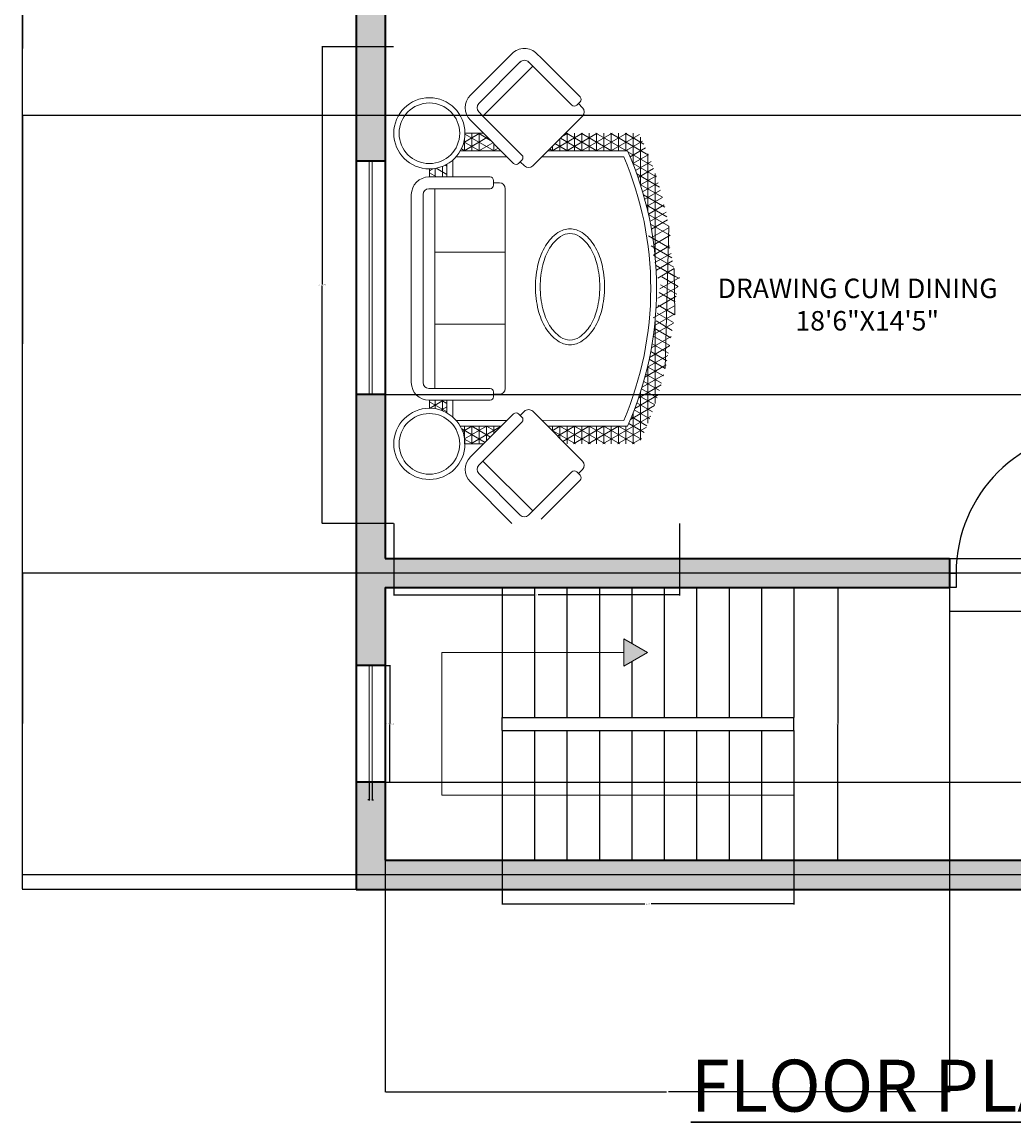
# Model space of a CAD drawing. Units: inches. Extents: x 5716 to 6907, y 12769 to 13594.
# Tile 1 of 17: x 5716 to 6022, y 12769 to 13109. Entities that reach past the tile are written whole.
import ezdxf

# ---------------------------------------------------------------- set-up
doc = ezdxf.new("R2010")
doc.units = ezdxf.units.IN
for name, color, linetype, lineweight in [('A-ANNO-DIMS', 2, 'Continuous', 18), ('A-ANNO-SYMB', 7, 'Continuous', 18), ('A-ANNO-TEXT', 7, 'Continuous', 30), ('A-AREA-IDEN', 7, 'Continuous', 18), ('A-DOOR', 4, 'Continuous', 25), ('A-FLOR-STRS', 7, 'Continuous', 25), ('A-FURN', 8, 'Continuous', 18), ('A-GLAZ', 4, 'Continuous', 18), ('A-WALL', 7, 'Continuous', 35), ('A-WALL-PATT', 252, 'Continuous', 13)]:
    doc.layers.add(name, color=color, linetype=linetype, lineweight=lineweight)
doc.styles.get("Standard").update_dxf_attribs({"font": 'arial.ttf'})
doc.dimstyles.get("Standard").update_dxf_attribs({"dimtxt": 0.18, "dimasz": 0.18, "dimexe": 0.18, "dimexo": 0.0625, "dimgap": 0.09, "dimtad": 0, "dimtih": 1, "dimtoh": 1, "dimdec": 4, "dimzin": 0, "dimdsep": 46, "dimtxsty": 'Standard', "dimcen": 0.09, "dimadec": 0, "dimazin": 0, "dimtfac": 1, "dimtdec": 4, "dimtofl": 0, "dimtmove": 0, "dimatfit": 3, "dimfxl": 1, "dimtolj": 1, "dimtzin": 0, "dimarcsym": 0})

# ---------------------------------------------------------------- blocks, each defined once
blk = doc.blocks.new('A$C7A76439A')
for p, q in [((2799, 2281.9), (1199, 2281.9)), ((1199, 2181.9), (2799, 2181.9)), ((948.9, 1978.3), (1035.6, 2128.3)), ((976.5, 2079.8), (1049, 2079.8)), ((1049, 2008), (979.5, 2128.3)), ((1049, 2128.3), (980.4, 2128.3)), ((1049, 2131.9), (1049, 2081.9)), ((1049, 2081.9), (1049, 1611.9)), ((1149, 1611.9), (1149, 2131.9)), ((2849, 2081.9), (1149, 2081.9)), ((1695.1, 2081.9), (1695.1, 1481.9)), ((2307.6, 2081.9), (2307.6, 1481.9)), ((2849, 2131.9), (2849, 1611.9)), ((2949, 2081.9), (2949, 2131.9)), ((3017.6, 2128.3), (2949, 2128.3)), ((2949, 2067.5), (2984.1, 2128.3)), ((2949, 1611.9), (2949, 2081.9)), ((2949, 2079.8), (3021.5, 2079.8)), ((2969.7, 1978.3), (3023.1, 2070.8)), ((3019.4, 2095.1), (3000.2, 2128.3)), ((940.7, 1978.3), (1049, 1978.3)), ((959.3, 2017.3), (1049, 2017.3)), ((993.9, 1978.3), (964, 2030.1)), ((1021.1, 1978.3), (1049, 2026.6)), ((2949, 2017.3), (3038.7, 2017.3)), ((2949, 1978.3), (3057.3, 1978.3)), ((3041.8, 1978.3), (3049.9, 1992.2)), ((877.3, 1467), (877.3, 1900.7)), ((905, 1928.3), (1049, 1928.3)), ((2949, 1928.3), (3093, 1928.3)), ((3120.6, 1900.7), (3120.6, 1467)), ((677.3, 1829.8), (827.3, 1829.8)), ((677.3, 1757.9), (717.8, 1828)), ((677.3, 1825.3), (677.3, 1667)), ((689.8, 1654.5), (804.6, 1853.3)), ((827.3, 1641.9), (719.7, 1828.3)), ((827.3, 1766.9), (782.7, 1844.2)), ((827.3, 1517), (827.3, 1865)), ((3170.6, 1865), (3170.6, 1517)), ((3170.6, 1826.4), (3187.7, 1856)), ((3170.6, 1701.4), (3247.3, 1834.3)), ((3286.4, 1632.8), (3170.6, 1833.2)), ((3170.6, 1829.8), (3268.5, 1829.8)), ((3170.6, 1576.4), (3314.4, 1825.4)), ((3320.6, 1698.4), (3241.3, 1835.9)), ((3320.6, 1823.4), (3319.5, 1825.3)), ((3320.6, 1667), (3320.6, 1825.3)), ((353.6, 1778.7), (0, 1425.1)), ((70.7, 1354.4), (424.3, 1708)), ((530.3, 1672.6), (495, 1708)), ((601, 1743.3), (565.7, 1778.7)), ((933.4, 1411), (601, 1743.3)), ((827.3, 1516.9), (677.3, 1776.7)), ((677.3, 1767.3), (827.3, 1767.3)), ((677.3, 1704.8), (827.3, 1704.8)), ((735.6, 1608.8), (827.3, 1767.7)), ((3064.6, 1411), (3396.9, 1743.3)), ((3170.6, 1767.3), (3320.6, 1767.3)), ((3240.6, 1587), (3170.6, 1708.2)), ((3170.6, 1704.8), (3320.6, 1704.8)), ((3260.3, 1606.7), (3320.6, 1711.2)), ((3396.9, 1743.3), (3432.3, 1778.7)), ((3467.6, 1672.6), (3503, 1708)), ((3927.3, 1354.4), (3573.7, 1708)), ((3644.4, 1778.7), (3998, 1425.1)), ((106.1, 1248.4), (530.3, 1672.6)), ((862.7, 1340.3), (530.3, 1672.6)), ((702.1, 1642.3), (827.3, 1642.3)), ((781.3, 1563), (827.3, 1642.7)), ((3135.3, 1340.3), (3467.6, 1672.6)), ((3891.9, 1248.4), (3467.6, 1672.6)), ((764.6, 1579.8), (827.3, 1579.8)), ((1099, 1581.9), (1079, 1581.9)), ((1119, 1581.9), (1099, 1581.9)), ((1099, 1581.9), (1099, 1531.9)), ((2899, 1581.9), (2879, 1581.9)), ((2919, 1581.9), (2899, 1581.9)), ((2899, 1581.9), (2899, 1531.9)), ((3194.9, 1541.3), (3170.6, 1583.2)), ((3170.6, 1579.8), (3233.4, 1579.8)), ((3170.6, 1517.3), (3170.9, 1517.3)), ((2849, 1481.9), (1149, 1481.9)), ((905.1, 1340.3), (933.4, 1368.6)), ((919.2, 1354.4), (954.6, 1319.1)), ((3078.7, 1354.4), (3043.4, 1319.1)), ((3092.9, 1340.3), (3064.6, 1368.6)), ((106.1, 1248.4), (70.7, 1283.7)), ((438.4, 916), (106.1, 1248.4)), ((530.3, 824.1), (954.6, 1248.4)), ((3467.6, 824.1), (3043.4, 1248.4)), ((3559.6, 916), (3891.9, 1248.4)), ((3891.9, 1248.4), (3927.3, 1283.7)), ((367.7, 845.3), (35.4, 1177.7)), ((877.3, 473.7), (879.6, 1173.4)), ((3120.6, 1171.1), (3120.6, 473.7)), ((3630.3, 845.3), (3962.6, 1177.7)), ((3998, 1213), (3962.6, 1177.7)), ((677.3, 882.9), (797.8, 1091.6)), ((827.3, 891.9), (743.4, 1037.2)), ((786, 1079.8), (827.3, 1079.8)), ((827.3, 1016.9), (789.2, 1083)), ((827.3, 440.9), (827.3, 1121.1)), ((3170.6, 1121.1), (3170.6, 440.9)), ((3170.6, 1076.4), (3187, 1104.8)), ((3320.6, 823.4), (3170.6, 1083.2)), ((3170.6, 1079.8), (3211.9, 1079.8)), ((3170.6, 951.4), (3232.8, 1059)), ((677.3, 757.9), (827.3, 1017.7)), ((677.3, 954.8), (827.3, 954.8)), ((827.3, 766.9), (697.7, 991.5)), ((723.5, 1017.3), (827.3, 1017.3)), ((3170.6, 1017.3), (3274.4, 1017.3)), ((3170.6, 826.4), (3278.5, 1013.2)), ((3170.6, 701.4), (3320.6, 961.2)), ((3320.6, 698.4), (3170.6, 958.2)), ((3170.6, 954.8), (3320.6, 954.8)), ((3320.6, 948.4), (3289.6, 1002.1)), ((410.1, 845.3), (438.4, 873.6)), ((424.3, 859.5), (459.6, 824.1)), ((827.3, 641.9), (677.3, 901.7)), ((677.3, 632.9), (827.3, 892.7)), ((677.3, 892.3), (827.3, 892.3)), ((3170.6, 892.3), (3320.6, 892.3)), ((3573.7, 859.5), (3538.4, 824.1)), ((3587.9, 845.3), (3559.6, 873.6)), ((677.3, 829.8), (827.3, 829.8)), ((827.3, 516.9), (677.3, 776.7)), ((677.3, 507.9), (827.3, 767.7)), ((677.3, 767.3), (827.3, 767.3)), ((3170.6, 576.4), (3320.6, 836.2)), ((3320.6, 573.4), (3170.6, 833.2)), ((3170.6, 829.8), (3320.6, 829.8)), ((3170.6, 767.3), (3320.6, 767.3)), ((677.3, 704.8), (827.3, 704.8)), ((3170.6, 451.4), (3320.6, 711.2)), ((3320.6, 448.4), (3170.6, 708.2)), ((3170.6, 704.8), (3320.6, 704.8)), ((913, 243.6), (677.3, 651.7)), ((677.3, 382.9), (827.3, 642.7)), ((677.3, 642.3), (827.3, 642.3)), ((677.3, 579.8), (827.3, 579.8)), ((3133.8, 262.7), (3320.6, 586.2)), ((3170.6, 642.3), (3320.6, 642.3)), ((3310.9, 340.3), (3170.6, 583.2)), ((3170.6, 579.8), (3320.6, 579.8)), ((819.1, 281.2), (677.3, 526.7)), ((677.3, 517.3), (827.3, 517.3)), ((716.8, 326.3), (827.3, 517.7)), ((3170.6, 517.3), (3320.6, 517.3)), ((677.3, 454.8), (827.3, 454.8)), ((722.3, 323.8), (677.3, 401.7)), ((677.3, 392.3), (944.2, 392.3)), ((774.1, 300.5), (849.6, 431.2)), ((832, 275.8), (907.7, 406.9)), ((1004.3, 210.4), (885.6, 415.9)), ((890.6, 252.2), (966.5, 383.7)), ((1093.3, 181.2), (979.2, 378.9)), ((2951, 196.1), (3067.5, 397.7)), ((3041.2, 227.3), (3162.5, 437.4)), ((3053.8, 392.3), (3320.6, 392.3)), ((3138.2, 264.4), (3062.4, 395.7)), ((3196.4, 288.6), (3120.8, 419.5)), ((3254, 313.9), (3170.6, 458.2)), ((3170.6, 454.8), (3320.6, 454.8)), ((3229.2, 302.8), (3320.6, 461.2)), ((709.3, 329.8), (1120.8, 329.8)), ((949.8, 229.8), (1026, 361.8)), ((1009.7, 208.6), (1086.2, 341.1)), ((1180.3, 155.6), (1070.1, 346.5)), ((1070.3, 188.5), (1147.1, 321.6)), ((1131.5, 169.6), (1208.8, 303.4)), ((1265.4, 133.2), (1158.6, 318.1)), ((1193.5, 151.9), (1271.2, 286.4)), ((1348.8, 113.7), (1245.1, 293.3)), ((2610.1, 105.5), (2712.4, 282.8)), ((2692.7, 123.6), (2797.9, 305.9)), ((2837, 161), (2759.6, 295.2)), ((2776.9, 144.5), (2885.5, 332.5)), ((2898.6, 179.3), (2821.6, 312.8)), ((2863, 168.6), (2975.2, 362.9)), ((2877.1, 329.8), (3288.7, 329.8)), ((2959.5, 198.9), (2882.9, 331.6)), ((3019.7, 219.6), (2943.4, 351.8)), ((3079.3, 241.4), (3003.3, 373.1)), ((852.7, 267.3), (1349.4, 267.3)), ((1020.7, 204.8), (1744.2, 204.8)), ((1256.2, 135.5), (1334.3, 270.8)), ((1319.6, 120.3), (1398.2, 256.5)), ((1430.6, 97), (1329.6, 271.9)), ((1383.7, 106.3), (1462.9, 243.6)), ((1510.9, 82.9), (1412.4, 253.6)), ((1448.6, 93.7), (1528.4, 232)), ((1589.9, 71.2), (1493.6, 238)), ((1514.2, 82.4), (1594.8, 221.9)), ((1580.6, 72.4), (1661.9, 213.2)), ((1705.7, 49.7), (1607.2, 220.4)), ((1643.3, 60.5), (1723.2, 198.8)), ((1784.6, 38), (1688.3, 204.8)), ((1709, 49.2), (1789.5, 188.7)), ((1852.3, 42.6), (1748.6, 222.2)), ((1934.2, 25.9), (1833.2, 200.8)), ((2100.1, 34.3), (2197.6, 203.1)), ((2234.3, 57.4), (2154.8, 195.2)), ((2179.8, 47.3), (2279.6, 220.1)), ((2298.8, 70.8), (2219.9, 207.5)), ((2253.8, 204.8), (2977.3, 204.8)), ((2260.9, 62.8), (2363.3, 240.1)), ((2362.6, 85.4), (2284.2, 221.1)), ((2343.5, 80.9), (2448.8, 263.2)), ((2452.3, 77.5), (2371.4, 217.6)), ((2518.3, 88.1), (2438.1, 227)), ((2449.3, 77), (2546.8, 245.8)), ((2583.5, 100.1), (2504, 237.9)), ((2529, 90), (2628.7, 262.8)), ((2648, 113.5), (2569, 250.2)), ((2711.7, 128.1), (2633.3, 263.8)), ((2648.6, 267.3), (3145.3, 267.3)), ((2774.7, 143.9), (2696.8, 278.8)), ((1319.6, 120.3), (2529, 90)), ((1775.4, 39.2), (1856.7, 180)), ((1887.2, 35.2), (1966.5, 172.4)), ((2014.5, 11.7), (1916, 182.4)), ((1952.1, 22.5), (2032, 160.9)), ((2093.4, 0), (1997.1, 166.8)), ((2017.8, 11.2), (2098.3, 150.7)), ((2084.2, 1.3), (2165.5, 142.1)), ((2169.1, 45.4), (2088.9, 184.3)), ((1775.4, 39.2), (2169.1, 45.4))]:
    blk.add_line(p, q)
for centre, radius in [((677.3, 2128.3), 303), ((677.3, 2128.3), 258), ((3320.6, 2128.3), 303), ((3320.6, 2128.3), 258)]:
    blk.add_circle(centre, radius)
for centre, radius, start, end in [((1199, 2131.9), 150, 90, 180), ((2799, 2131.9), 150, 0, 90), ((1199, 2131.9), 50, 90, 180), ((2799, 2131.9), 50, 0, 90), ((459.6, 1672.6), 150, 45, 135), ((3538.4, 1672.6), 150, 45, 135), ((459.6, 1672.6), 50, 45, 135), ((3538.4, 1672.6), 50, 45, 135), ((1079, 1611.9), 30, 180, 270), ((1119, 1611.9), 30, 270, 0), ((2879, 1611.9), 30, 180, 270), ((2919, 1611.9), 30, 270, 0), ((1149, 1531.9), 50, 180, 270), ((2849, 1531.9), 50, 270, 0), ((912.2, 1389.8), 30, 315, 45), ((3085.8, 1389.8), 30, 135, 225), ((3891.9, 1319.1), 150, 315, 45), ((106.1, 1319.1), 50, 135, 225), ((883.9, 1361.5), 30, 225, 315), ((919.2, 1283.7), 50, 315, 45), ((3078.7, 1283.7), 50, 135, 225), ((3114.1, 1361.5), 30, 225, 315), ((3891.9, 1319.1), 50, 315, 45), ((2014.2, 399.9), 825, 90, 103.86382), ((2014.2, 399.9), 825, 76.13618, 90), ((1850.9, 827.5), 362.5, 120.78817, 145.1939), ((1949.5, 662.2), 555, 103.86382, 120.78817), ((1949.5, 662.2), 515, 103.86382, 120.78817), ((2014.2, 399.9), 785, 90, 103.86382), ((2014.2, 399.9), 785, 76.13618, 90), ((2078.9, 662.2), 515, 59.21183, 76.13618), ((2078.9, 662.2), 555, 59.21183, 76.13618), ((2177.4, 827.5), 362.5, 34.8061, 59.21183), ((1702, 931.1), 181, 145.1939, 180), ((1850.9, 827.5), 322.5, 120.78817, 145.1939), ((2177.4, 827.5), 322.5, 34.8061, 59.21183), ((2326.4, 931.1), 181, 0, 34.8061), ((1702, 931.1), 141, 145.1939, 180), ((2326.4, 931.1), 141, 0, 34.8061), ((388.9, 866.5), 30, 225, 315), ((417.2, 894.8), 30, 315, 45), ((1702, 931.1), 181, 180, 214.8061), ((1702, 931.1), 141, 180, 214.8061), ((1850.9, 1034.6), 322.5, 214.8061, 239.21183), ((2177.4, 1034.6), 322.5, 300.78817, 325.1939), ((2326.4, 931.1), 141, 325.1939, 0), ((2326.4, 931.1), 181, 325.1939, 0), ((3580.8, 894.8), 30, 135, 225), ((3609.1, 866.5), 30, 225, 315), ((495, 859.5), 50, 225, 315), ((1850.9, 1034.6), 362.5, 214.8061, 239.21183), ((1949.5, 1200), 515, 239.21183, 256.13618), ((2078.9, 1200), 515, 283.86382, 300.78817), ((2177.4, 1034.6), 362.5, 300.78817, 325.1939), ((3503, 859.5), 50, 225, 315), ((1949.5, 1200), 555, 239.21183, 256.13618), ((2014.2, 1462.2), 825, 256.13618, 270), ((2014.2, 1462.2), 785, 256.13618, 270), ((2014.2, 1462.2), 785, 270, 283.86382), ((2014.2, 1462.2), 825, 270, 283.86382), ((2078.9, 1200), 555, 283.86382, 300.78817), ((1999, 3092.2), 2848.7, 246.81236, 293.18764), ((1999, 3092.2), 2898.7, 246.15892, 293.84108)]:
    blk.add_arc(centre, radius, start, end)
blk = doc.blocks.new('DOOR-SWING-48IN')
for p, q in [((-2, 43.95), (-2, 0)), ((0, 44), (0, 0)), ((-46, 0), (-44, 0)), ((-44, 0), (-44, -4.5)), ((0, 0), (-2, 0)), ((2, 0), (0, 0)), ((0, 0), (0, -4.5)), ((-44, -4.5), (-46, -4.5)), ((0, -4.5), (2, -4.5))]:
    blk.add_line(p, q)
blk.add_arc((0, 0), 44, 90, 180)
blk = doc.blocks.new('WIN-GLAZING-72IN')
for p, q in [((0, 0), (0, -72)), ((1, 0), (1, -72))]:
    blk.add_line(p, q)
blk = doc.blocks.new('WIN-GLAZING-36IN')
for p, q in [((0, 0), (0, 36)), ((1, 0), (1, 36))]:
    blk.add_line(p, q)
blk = doc.blocks.new('STAIR-RETURN-FLIGHT')
for p, q in [((0, 84), (0, 44)), ((10, 84), (10, 44)), ((20, 84), (20, 44)), ((30, 84), (30, 44)), ((40, 84), (40, 66.79)), ((50, 84), (50, 44)), ((60, 84), (60, 44)), ((70, 84), (70, 44)), ((80, 84), (80, 44)), ((90, 84), (90, 44)), ((40, 61.21), (40, 44)), ((0, 44), (90, 44)), ((0, 40), (0, 44)), ((90, 40), (90, 44)), ((0, 40), (90, 40)), ((0, 40), (0, 0)), ((10, 40), (10, 0)), ((20, 40), (20, 0)), ((30, 40), (30, 0)), ((40, 40), (40, 0)), ((50, 40), (50, 0)), ((60, 40), (60, 0)), ((70, 40), (70, 0)), ((80, 40), (80, 0)), ((90, 40), (90, 0))]:
    blk.add_line(p, q)
blk = doc.blocks.new('*D33')
at = {"layer": 'A-ANNO-DIMS', "color": 0, "lineweight": -2, "transparency": 16777216}
for p, q in [((5830.57, 13100.85), (5808.41, 13100.85)), ((5808.59, 13100.67), (5808.59, 13027.58)), ((5808.59, 12954.12), (5808.59, 13027.21)), ((5830.57, 12953.94), (5808.41, 12953.94))]:
    blk.add_line(p, q, dxfattribs=at)
at = {"layer": 'A-ANNO-DIMS', "color": 0, "transparency": 16777216}
for points in [[(5808.56, 13100.67), (5808.62, 13100.67), (5808.59, 13100.85)], [(5808.56, 12954.12), (5808.62, 12954.12), (5808.59, 12953.94)]]:
    blk.add_solid(points, dxfattribs=at)
at = {"layer": 'Defpoints', "color": 0, "transparency": 16777216}
for p in [(5808.59, 13100.85), (5830.63, 13100.85), (5830.63, 12953.94)]:
    blk.add_point(p, dxfattribs=at)
at = {"layer": 'A-ANNO-DIMS', "color": 0, "transparency": 16777216, "insert": (5808.59, 13027.4), "char_height": 0.18, "attachment_point": 5}
blk.add_mtext('\\A1;SOFA GROUP 147 TYP.', dxfattribs=at)
blk = doc.blocks.new('*D34')
at = {"layer": 'A-ANNO-DIMS', "color": 0, "lineweight": -2, "transparency": 16777216}
for p, q in [((5830.63, 12953.88), (5830.63, 12931.72)), ((5918.69, 12953.88), (5918.69, 12931.72)), ((5830.81, 12931.9), (5874.13, 12931.9)), ((5918.51, 12931.9), (5875.19, 12931.9))]:
    blk.add_line(p, q, dxfattribs=at)
at = {"layer": 'A-ANNO-DIMS', "color": 0, "transparency": 16777216}
for points in [[(5830.81, 12931.93), (5830.81, 12931.87), (5830.63, 12931.9)], [(5918.51, 12931.93), (5918.51, 12931.87), (5918.69, 12931.9)]]:
    blk.add_solid(points, dxfattribs=at)
at = {"layer": 'Defpoints', "color": 0, "transparency": 16777216}
for p in [(5830.63, 12953.94), (5918.69, 12953.94), (5830.63, 12931.9)]:
    blk.add_point(p, dxfattribs=at)
at = {"layer": 'A-ANNO-DIMS', "color": 0, "transparency": 16777216, "insert": (5874.66, 12931.9), "char_height": 0.18, "attachment_point": 5}
blk.add_mtext('\\A1;88 TYP.', dxfattribs=at)
blk = doc.blocks.new('*D42')
at = {"layer": 'A-ANNO-DIMS', "color": 0, "lineweight": -2, "transparency": 16777216}
for p, q in [((6002.02, 12934.09), (6002.02, 12926.69)), ((6050.02, 12934.09), (6050.02, 12926.69)), ((6002.2, 12926.87), (6025.49, 12926.87)), ((6049.84, 12926.87), (6026.55, 12926.87))]:
    blk.add_line(p, q, dxfattribs=at)
at = {"layer": 'A-ANNO-DIMS', "color": 0, "transparency": 16777216}
for points in [[(6002.2, 12926.9), (6002.2, 12926.84), (6002.02, 12926.87)], [(6049.84, 12926.9), (6049.84, 12926.84), (6050.02, 12926.87)]]:
    blk.add_solid(points, dxfattribs=at)
at = {"layer": 'Defpoints', "color": 0, "transparency": 16777216}
for p in [(6002.02, 12934.15), (6050.02, 12934.15), (6050.02, 12926.87)]:
    blk.add_point(p, dxfattribs=at)
at = {"layer": 'A-ANNO-DIMS', "color": 0, "transparency": 16777216, "insert": (6026.02, 12926.87), "char_height": 0.18, "attachment_point": 5}
blk.add_mtext('\\A1;48 TYP.', dxfattribs=at)
blk = doc.blocks.new('*D43')
at = {"layer": 'A-ANNO-DIMS', "color": 0, "lineweight": -2, "transparency": 16777216}
for p, q in [((5824.09, 12910.15), (5829.6, 12910.15)), ((5829.42, 12909.97), (5829.42, 12892.33)), ((5829.42, 12874.33), (5829.42, 12891.97)), ((5824.09, 12874.15), (5829.6, 12874.15))]:
    blk.add_line(p, q, dxfattribs=at)
at = {"layer": 'A-ANNO-DIMS', "color": 0, "transparency": 16777216}
for points in [[(5829.39, 12909.97), (5829.45, 12909.97), (5829.42, 12910.15)], [(5829.39, 12874.33), (5829.45, 12874.33), (5829.42, 12874.15)]]:
    blk.add_solid(points, dxfattribs=at)
at = {"layer": 'Defpoints', "color": 0, "transparency": 16777216}
for p in [(5824.02, 12910.15), (5829.42, 12910.15), (5824.02, 12874.15)]:
    blk.add_point(p, dxfattribs=at)
at = {"layer": 'A-ANNO-DIMS', "color": 0, "transparency": 16777216, "insert": (5829.42, 12892.15), "char_height": 0.18, "attachment_point": 5}
blk.add_mtext('\\A1;STAIR WINDOW 36 TYP.', dxfattribs=at)
blk = doc.blocks.new('*D44')
at = {"layer": 'A-ANNO-DIMS', "color": 0, "lineweight": -2, "transparency": 16777216}
for p, q in [((5823.02, 12874.09), (5823.02, 12868.57)), ((5824.02, 12874.09), (5824.02, 12868.57)), ((5822.84, 12868.75), (5822.66, 12868.75)), ((5824.2, 12868.75), (5824.38, 12868.75))]:
    blk.add_line(p, q, dxfattribs=at)
at = {"layer": 'A-ANNO-DIMS', "color": 0, "transparency": 16777216}
for points in [[(5822.84, 12868.78), (5822.84, 12868.72), (5823.02, 12868.75)], [(5824.2, 12868.78), (5824.2, 12868.72), (5824.02, 12868.75)]]:
    blk.add_solid(points, dxfattribs=at)
at = {"layer": 'Defpoints', "color": 0, "transparency": 16777216}
for p in [(5823.02, 12874.15), (5824.02, 12874.15), (5824.02, 12868.75)]:
    blk.add_point(p, dxfattribs=at)
at = {"layer": 'A-ANNO-DIMS', "color": 0, "transparency": 16777216, "insert": (5823.52, 12868.75), "char_height": 0.18, "attachment_point": 5}
blk.add_mtext('\\A1;1 TYP.', dxfattribs=at)
blk = doc.blocks.new('*D45')
at = {"layer": 'A-ANNO-DIMS', "color": 0, "lineweight": -2, "transparency": 16777216}
for p, q in [((5864.02, 12850.09), (5864.02, 12836.47)), ((5954.02, 12850.09), (5954.02, 12836.47)), ((5864.2, 12836.65), (5908.09, 12836.65)), ((5953.84, 12836.65), (5909.96, 12836.65))]:
    blk.add_line(p, q, dxfattribs=at)
at = {"layer": 'A-ANNO-DIMS', "color": 0, "transparency": 16777216}
for points in [[(5864.2, 12836.68), (5864.2, 12836.62), (5864.02, 12836.65)], [(5953.84, 12836.68), (5953.84, 12836.62), (5954.02, 12836.65)]]:
    blk.add_solid(points, dxfattribs=at)
at = {"layer": 'Defpoints', "color": 0, "transparency": 16777216}
for p in [(5864.02, 12850.15), (5954.02, 12850.15), (5954.02, 12836.65)]:
    blk.add_point(p, dxfattribs=at)
at = {"layer": 'A-ANNO-DIMS', "color": 0, "transparency": 16777216, "insert": (5909.02, 12836.65), "char_height": 0.18, "attachment_point": 5}
blk.add_mtext('\\A1;STAIR 90 TYP.', dxfattribs=at)
blk = doc.blocks.new('*D46')
at = {"layer": 'A-ANNO-DIMS', "color": 0, "lineweight": -2, "transparency": 16777216}
for p, q in [((5954.09, 12934.15), (5967.7, 12934.15)), ((5967.52, 12933.97), (5967.52, 12892.33)), ((5967.52, 12850.33), (5967.52, 12891.97)), ((5954.09, 12850.15), (5967.7, 12850.15))]:
    blk.add_line(p, q, dxfattribs=at)
at = {"layer": 'A-ANNO-DIMS', "color": 0, "transparency": 16777216}
for points in [[(5967.49, 12933.97), (5967.55, 12933.97), (5967.52, 12934.15)], [(5967.49, 12850.33), (5967.55, 12850.33), (5967.52, 12850.15)]]:
    blk.add_solid(points, dxfattribs=at)
at = {"layer": 'Defpoints', "color": 0, "transparency": 16777216}
for p in [(5954.02, 12934.15), (5967.52, 12934.15), (5954.02, 12850.15)]:
    blk.add_point(p, dxfattribs=at)
at = {"layer": 'A-ANNO-DIMS', "color": 0, "transparency": 16777216, "insert": (5967.52, 12892.15), "char_height": 0.18, "attachment_point": 5}
blk.add_mtext('\\A1;84 TYP.', dxfattribs=at)
blk = doc.blocks.new('*D50')
at = {"layer": 'A-ANNO-DIMS', "color": 0, "lineweight": -2, "transparency": 16777216}
for p, q in [((5818.96, 13440.15), (5716.04, 13440.15)), ((5716.22, 13439.97), (5716.22, 13140.83)), ((5716.22, 12841.33), (5716.22, 13140.47)), ((5818.96, 12841.15), (5716.04, 12841.15))]:
    blk.add_line(p, q, dxfattribs=at)
at = {"layer": 'A-ANNO-DIMS', "color": 0, "transparency": 16777216}
for points in [[(5716.19, 13439.97), (5716.25, 13439.97), (5716.22, 13440.15)], [(5716.19, 12841.33), (5716.25, 12841.33), (5716.22, 12841.15)]]:
    blk.add_solid(points, dxfattribs=at)
at = {"layer": 'Defpoints', "color": 0, "transparency": 16777216}
for p in [(5716.22, 13440.15), (5819.02, 13440.15), (5819.02, 12841.15)]:
    blk.add_point(p, dxfattribs=at)
at = {"layer": 'A-ANNO-DIMS', "color": 0, "transparency": 16777216, "insert": (5716.22, 13140.65), "char_height": 0.18, "attachment_point": 5}
blk.add_mtext('\\A1;599', dxfattribs=at)
blk = doc.blocks.new('*D52')
at = {"layer": 'A-ANNO-DIMS', "color": 0, "lineweight": -2, "transparency": 16777216}
for p, q in [((6267.34, 13440.15), (5716.04, 13440.15)), ((5716.22, 13439.97), (5716.22, 13140.83)), ((5716.22, 12841.33), (5716.22, 13140.47)), ((6267.34, 12841.15), (5716.04, 12841.15))]:
    blk.add_line(p, q, dxfattribs=at)
at = {"layer": 'A-ANNO-DIMS', "color": 0, "transparency": 16777216}
for points in [[(5716.19, 13439.97), (5716.25, 13439.97), (5716.22, 13440.15)], [(5716.19, 12841.33), (5716.25, 12841.33), (5716.22, 12841.15)]]:
    blk.add_solid(points, dxfattribs=at)
at = {"layer": 'Defpoints', "color": 0, "transparency": 16777216}
for p in [(6267.41, 13440.15), (5716.22, 12841.15), (6267.41, 12841.15)]:
    blk.add_point(p, dxfattribs=at)
at = {"layer": 'A-ANNO-DIMS', "color": 0, "transparency": 16777216, "insert": (5716.22, 13140.65), "char_height": 0.18, "attachment_point": 5}
blk.add_mtext('\\A1;599', dxfattribs=at)
blk = doc.blocks.new('*D62')
at = {"layer": 'A-ANNO-DIMS', "color": 0, "lineweight": -2, "transparency": 16777216}
for p, q in [((6736.67, 13120.65), (5716.04, 13120.65)), ((5716.22, 13120.47), (5716.22, 13100.33)), ((5716.22, 13079.83), (5716.22, 13099.97)), ((6736.67, 13079.65), (5716.04, 13079.65))]:
    blk.add_line(p, q, dxfattribs=at)
at = {"layer": 'A-ANNO-DIMS', "color": 0, "transparency": 16777216}
for points in [[(5716.19, 13120.47), (5716.25, 13120.47), (5716.22, 13120.65)], [(5716.19, 13079.83), (5716.25, 13079.83), (5716.22, 13079.65)]]:
    blk.add_solid(points, dxfattribs=at)
at = {"layer": 'Defpoints', "color": 0, "transparency": 16777216}
for p in [(6736.73, 13120.65), (5716.22, 13079.65), (6736.73, 13079.65)]:
    blk.add_point(p, dxfattribs=at)
at = {"layer": 'A-ANNO-DIMS', "color": 0, "transparency": 16777216, "insert": (5716.22, 13100.15), "char_height": 0.18, "attachment_point": 5}
blk.add_mtext('\\A1;41', dxfattribs=at)
blk = doc.blocks.new('*D63')
at = {"layer": 'A-ANNO-DIMS', "color": 0, "lineweight": -2, "transparency": 16777216}
for p, q in [((6736.67, 13079.65), (5716.04, 13079.65)), ((5716.22, 13079.47), (5716.22, 13009.33)), ((5716.22, 12938.83), (5716.22, 13008.97)), ((6736.67, 12938.65), (5716.04, 12938.65))]:
    blk.add_line(p, q, dxfattribs=at)
at = {"layer": 'A-ANNO-DIMS', "color": 0, "transparency": 16777216}
for points in [[(5716.19, 13079.47), (5716.25, 13079.47), (5716.22, 13079.65)], [(5716.19, 12938.83), (5716.25, 12938.83), (5716.22, 12938.65)]]:
    blk.add_solid(points, dxfattribs=at)
at = {"layer": 'Defpoints', "color": 0, "transparency": 16777216}
for p in [(6736.73, 13079.65), (5716.22, 12938.65), (6736.73, 12938.65)]:
    blk.add_point(p, dxfattribs=at)
at = {"layer": 'A-ANNO-DIMS', "color": 0, "transparency": 16777216, "insert": (5716.22, 13009.15), "char_height": 0.18, "attachment_point": 5}
blk.add_mtext('\\A1;141', dxfattribs=at)
blk = doc.blocks.new('*D64')
at = {"layer": 'A-ANNO-DIMS', "color": 0, "lineweight": -2, "transparency": 16777216}
for p, q in [((6736.67, 12938.65), (5716.04, 12938.65)), ((5716.22, 12938.47), (5716.22, 12892.33)), ((5716.22, 12845.83), (5716.22, 12891.97)), ((6736.67, 12845.65), (5716.04, 12845.65))]:
    blk.add_line(p, q, dxfattribs=at)
at = {"layer": 'A-ANNO-DIMS', "color": 0, "transparency": 16777216}
for points in [[(5716.19, 12938.47), (5716.25, 12938.47), (5716.22, 12938.65)], [(5716.19, 12845.83), (5716.25, 12845.83), (5716.22, 12845.65)]]:
    blk.add_solid(points, dxfattribs=at)
at = {"layer": 'Defpoints', "color": 0, "transparency": 16777216}
for p in [(6736.73, 12938.65), (5716.22, 12845.65), (6736.73, 12845.65)]:
    blk.add_point(p, dxfattribs=at)
at = {"layer": 'A-ANNO-DIMS', "color": 0, "transparency": 16777216, "insert": (5716.22, 12892.15), "char_height": 0.18, "attachment_point": 5}
blk.add_mtext('\\A1;93', dxfattribs=at)
blk = doc.blocks.new('*D66')
at = {"layer": 'A-ANNO-DIMS', "color": 0, "lineweight": -2, "transparency": 16777216}
for p, q in [((6002.02, 12934.09), (6002.02, 12778.62)), ((5828.02, 12850.09), (5828.02, 12778.62)), ((5828.2, 12778.8), (5914.74, 12778.8)), ((6001.84, 12778.8), (5915.3, 12778.8))]:
    blk.add_line(p, q, dxfattribs=at)
at = {"layer": 'A-ANNO-DIMS', "color": 0, "transparency": 16777216}
for points in [[(5828.2, 12778.83), (5828.2, 12778.77), (5828.02, 12778.8)], [(6001.84, 12778.83), (6001.84, 12778.77), (6002.02, 12778.8)]]:
    blk.add_solid(points, dxfattribs=at)
at = {"layer": 'Defpoints', "color": 0, "transparency": 16777216}
for p in [(6002.02, 12934.15), (5828.02, 12850.15), (6002.02, 12778.8)]:
    blk.add_point(p, dxfattribs=at)
at = {"layer": 'A-ANNO-DIMS', "color": 0, "transparency": 16777216, "insert": (5915.02, 12778.8), "char_height": 0.18, "attachment_point": 5}
blk.add_mtext('\\A1;174', dxfattribs=at)
blk = doc.blocks.new('*D67')
at = {"layer": 'A-ANNO-DIMS', "color": 0, "lineweight": -2, "transparency": 16777216}
for p, q in [((5819.09, 12874.15), (6907.26, 12874.15)), ((6907.08, 12873.97), (6907.08, 12857.83)), ((6907.08, 12841.33), (6907.08, 12857.47)), ((5819.09, 12841.15), (6907.26, 12841.15))]:
    blk.add_line(p, q, dxfattribs=at)
at = {"layer": 'A-ANNO-DIMS', "color": 0, "transparency": 16777216}
for points in [[(6907.05, 12873.97), (6907.11, 12873.97), (6907.08, 12874.15)], [(6907.05, 12841.33), (6907.11, 12841.33), (6907.08, 12841.15)]]:
    blk.add_solid(points, dxfattribs=at)
at = {"layer": 'Defpoints', "color": 0, "transparency": 16777216}
for p in [(5819.02, 12874.15), (6907.08, 12874.15), (5819.02, 12841.15)]:
    blk.add_point(p, dxfattribs=at)
at = {"layer": 'A-ANNO-DIMS', "color": 0, "transparency": 16777216, "insert": (6907.08, 12857.65), "char_height": 0.18, "attachment_point": 5}
blk.add_mtext('\\A1;33', dxfattribs=at)
blk = doc.blocks.new('*D68')
at = {"layer": 'A-ANNO-DIMS', "color": 0, "lineweight": -2, "transparency": 16777216}
for p, q in [((5828.09, 12993.65), (6907.26, 12993.65)), ((6907.08, 12993.47), (6907.08, 12968.58)), ((6907.08, 12943.33), (6907.08, 12968.22)), ((5828.09, 12943.15), (6907.26, 12943.15))]:
    blk.add_line(p, q, dxfattribs=at)
at = {"layer": 'A-ANNO-DIMS', "color": 0, "transparency": 16777216}
for points in [[(6907.05, 12993.47), (6907.11, 12993.47), (6907.08, 12993.65)], [(6907.05, 12943.33), (6907.11, 12943.33), (6907.08, 12943.15)]]:
    blk.add_solid(points, dxfattribs=at)
at = {"layer": 'Defpoints', "color": 0, "transparency": 16777216}
for p in [(5828.02, 12993.65), (6907.08, 12993.65), (5828.02, 12943.15)]:
    blk.add_point(p, dxfattribs=at)
at = {"layer": 'A-ANNO-DIMS', "color": 0, "transparency": 16777216, "insert": (6907.08, 12968.4), "char_height": 0.18, "attachment_point": 5}
blk.add_mtext('\\A1;50.5', dxfattribs=at)

msp = doc.modelspace()

# ---------------------------------------------------------------- hatches: boundary and pattern name
at = {"layer": 'A-ANNO-SYMB'}
h = msp.add_hatch(color=256, dxfattribs=at)
h.dxf.hatch_style = 1
h.paths.add_polyline_path([(5901.6, 12909.96), (5908.86, 12914.15), (5901.6, 12918.34)])
at = {"layer": 'A-WALL-PATT'}
h = msp.add_hatch(color=256, dxfattribs=at)
h.dxf.hatch_style = 1
h.paths.add_polyline_path([(5900.02, 13125.15), (5828.02, 13125.15), (5828.02, 13149.15), (5819.02, 13149.15), (5819.02, 13065.65), (5828.02, 13065.65), (5828.02, 13116.15), (5900.02, 13116.15)])
h = msp.add_hatch(color=256, dxfattribs=at)
h.dxf.hatch_style = 1
h.paths.add_polyline_path([(6002.02, 12943.15), (5828.02, 12943.15), (5828.02, 12993.65), (5819.02, 12993.65), (5819.02, 12910.15), (5828.02, 12910.15), (5828.02, 12934.15), (6002.02, 12934.15)])
h = msp.add_hatch(color=256, dxfattribs=at)
h.dxf.hatch_style = 1
h.paths.add_polyline_path([(6059.02, 12862.15), (6050.02, 12862.15), (6050.02, 12850.15), (5828.02, 12850.15), (5828.02, 12874.15), (5819.02, 12874.15), (5819.02, 12841.15), (6059.02, 12841.15)])

# ---------------------------------------------------------------- linework, layer by layer
at = {"layer": 'A-ANNO-SYMB'}
for p, q in [((5845.47, 12870.15), (5845.47, 12914.15)), ((5901.6, 12914.15), (5845.47, 12914.15)), ((5954.02, 12870.15), (5845.47, 12870.15))]:
    msp.add_line(p, q, dxfattribs=at)
msp.add_lwpolyline([(5908.86, 12914.15), (5901.6, 12918.34), (5901.6, 12909.96)], close=True, dxfattribs=at)
at = {"layer": 'A-WALL'}
for p, q in [((5819.02, 13440.15), (5819.02, 12841.15)), ((5828.02, 13116.15), (5828.02, 12943.15)), ((5828.02, 13065.65), (5819.02, 13065.65)), ((5828.02, 12993.65), (5819.02, 12993.65)), ((5828.02, 12943.15), (6002.02, 12943.15)), ((6002.02, 12943.15), (6002.02, 12934.15)), ((5828.02, 12934.15), (6002.02, 12934.15)), ((5828.02, 12934.15), (5828.02, 12850.15)), ((5828.02, 12910.15), (5819.02, 12910.15)), ((5828.02, 12874.15), (5819.02, 12874.15)), ((5828.02, 12850.15), (6050.02, 12850.15)), ((5819.02, 12841.15), (6059.02, 12841.15))]:
    msp.add_line(p, q, dxfattribs=at)

# ---------------------------------------------------------------- block references
at = {"layer": 'A-DOOR'}
msp.add_blockref('DOOR-SWING-48IN', (6048.02, 12938.65), dxfattribs=at)
at = {"layer": 'A-FLOR-STRS'}
msp.add_blockref('STAIR-RETURN-FLIGHT', (5864.02, 12850.15), dxfattribs=at)
at = {"layer": 'A-FURN', "xscale": 0.0362164969968974, "yscale": 0.0362164969968974, "zscale": 0.0362164969968974, "rotation": 90}
msp.add_blockref('A$C7A76439A', (5918.69, 12953.94), dxfattribs=at)
at = {"layer": 'A-GLAZ'}
for name, p in [('WIN-GLAZING-72IN', (5823.02, 13065.65)), ('WIN-GLAZING-36IN', (5823.02, 12874.15))]:
    msp.add_blockref(name, p, dxfattribs=at)

# ---------------------------------------------------------------- texts
at = {"layer": 'A-ANNO-TEXT', "insert": (5922.18, 12788.65), "char_height": 16, "attachment_point": 1}
msp.add_mtext_dynamic_manual_height_columns('{\\LFLOOR PLAN}', width=852.8728, gutter_width=12.5, heights=[0], dxfattribs=at)
at = {"layer": 'A-AREA-IDEN', "insert": (5930.49, 13029.41), "char_height": 6, "attachment_point": 1}
msp.add_mtext_dynamic_manual_height_columns('DRAWING CUM DINING\\P^I18\'6"X14\'5"', width=158.347, gutter_width=12.5, heights=[0], dxfattribs=at)

# ---------------------------------------------------------------- dimensions: what is measured, and where the dimension line sits
at = {"layer": 'A-ANNO-DIMS'}
for base, p1, p2, override, picture, middle in [((5716.22, 13440.15), (5819.02, 12841.15), (5819.02, 13440.15), {"dimdec": 0, "dimlfac": 1, "dimrnd": 0, "dimzin": 0, "dimdsep": 46, "dimlunit": 2}, '*D50', (5716.22, 13140.65)), ((5716.22, 12841.15), (6267.41, 13440.15), (6267.41, 12841.15), {"dimdec": 0, "dimlfac": 1, "dimrnd": 0, "dimzin": 0, "dimdsep": 46, "dimlunit": 2}, '*D52', (5716.22, 13140.65)), ((5716.22, 13079.65), (6736.73, 13120.65), (6736.73, 13079.65), {"dimdec": 0, "dimlfac": 1, "dimrnd": 0, "dimzin": 0, "dimdsep": 46, "dimlunit": 2}, '*D62', (5716.22, 13100.15)), ((5716.22, 12938.65), (6736.73, 13079.65), (6736.73, 12938.65), {"dimdec": 0, "dimlfac": 1, "dimrnd": 0, "dimzin": 0, "dimdsep": 46, "dimlunit": 2}, '*D63', (5716.22, 13009.15)), ((6907.08, 12993.65), (5828.02, 12943.15), (5828.02, 12993.65), {"dimdec": 1, "dimlfac": 1, "dimrnd": 0, "dimzin": 0, "dimdsep": 46, "dimlunit": 2}, '*D68', (6907.08, 12968.4)), ((5716.22, 12845.65), (6736.73, 12938.65), (6736.73, 12845.65), {"dimdec": 0, "dimlfac": 1, "dimrnd": 0, "dimzin": 0, "dimdsep": 46, "dimlunit": 2}, '*D64', (5716.22, 12892.15)), ((6907.08, 12874.15), (5819.02, 12841.15), (5819.02, 12874.15), {"dimdec": 0, "dimlfac": 1, "dimrnd": 0, "dimzin": 0, "dimdsep": 46, "dimlunit": 2}, '*D67', (6907.08, 12857.65))]:
    dim = msp.add_linear_dim(base=base, p1=p1, p2=p2, angle=90, dimstyle='Standard', override=override, dxfattribs=at)
    dim.commit()
    dim.dimension.update_dxf_attribs({"geometry": picture, "text_midpoint": middle})
for base, p1, p2, angle, text, picture, middle in [((5808.59, 13100.85), (5830.63, 12953.94), (5830.63, 13100.85), 90, 'SOFA GROUP <> TYP.', '*D33', (5808.59, 13027.4)), ((5830.63, 12931.9), (5918.69, 12953.94), (5830.63, 12953.94), 180, '<> TYP.', '*D34', (5874.66, 12931.9)), ((5967.52, 12934.15), (5954.02, 12850.15), (5954.02, 12934.15), 90, '<> TYP.', '*D46', (5967.52, 12892.15)), ((5829.42, 12910.15), (5824.02, 12874.15), (5824.02, 12910.15), 90, 'STAIR WINDOW <> TYP.', '*D43', (5829.42, 12892.15))]:
    dim = msp.add_linear_dim(base=base, p1=p1, p2=p2, angle=angle, text=text, dimstyle='Standard', override={"dimdec": 0, "dimlfac": 1, "dimrnd": 0, "dimzin": 0, "dimdsep": 46, "dimlunit": 2}, dxfattribs=at)
    dim.commit()
    dim.dimension.update_dxf_attribs({"geometry": picture, "text_midpoint": middle})
dim = msp.add_linear_dim(base=(6002.02, 12778.8), p1=(5828.02, 12850.15), p2=(6002.02, 12934.15), dimstyle='Standard', override={"dimdec": 0, "dimlfac": 1, "dimrnd": 0, "dimzin": 0, "dimdsep": 46, "dimlunit": 2}, dxfattribs=at)
dim.commit()
dim.dimension.update_dxf_attribs({"geometry": '*D66', "text_midpoint": (5915.02, 12778.8)})
for base, p1, p2, text, picture, middle in [((6050.02, 12926.87), (6002.02, 12934.15), (6050.02, 12934.15), '<> TYP.', '*D42', (6026.02, 12926.87)), ((5824.02, 12868.75), (5823.02, 12874.15), (5824.02, 12874.15), '<> TYP.', '*D44', (5823.52, 12868.75)), ((5954.02, 12836.65), (5864.02, 12850.15), (5954.02, 12850.15), 'STAIR <> TYP.', '*D45', (5909.02, 12836.65))]:
    dim = msp.add_linear_dim(base=base, p1=p1, p2=p2, text=text, dimstyle='Standard', override={"dimdec": 0, "dimlfac": 1, "dimrnd": 0, "dimzin": 0, "dimdsep": 46, "dimlunit": 2}, dxfattribs=at)
    dim.commit()
    dim.dimension.update_dxf_attribs({"geometry": picture, "text_midpoint": middle})

doc.saveas('drawing.dxf')
